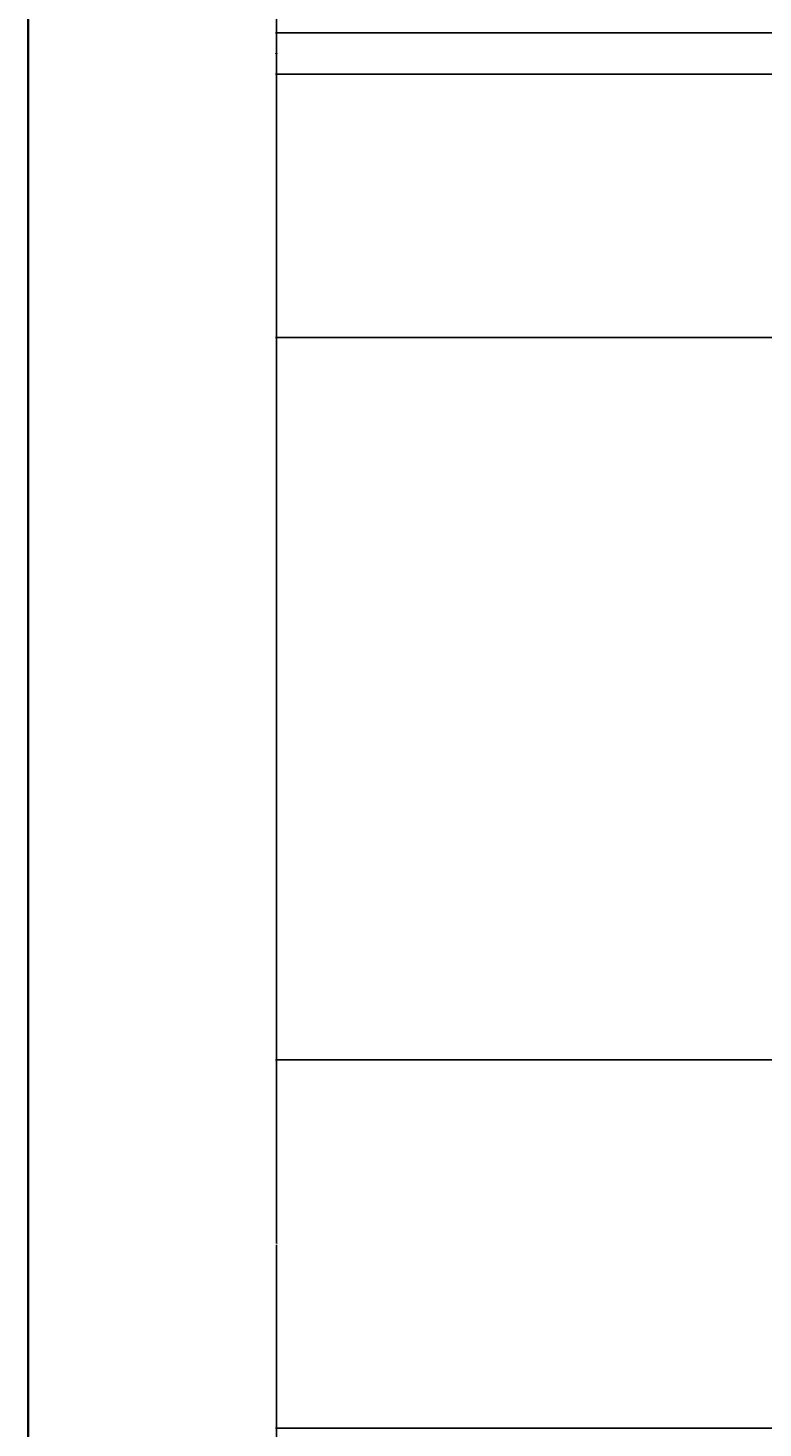
# Model space of a CAD drawing. Units: inches. Extents: x 1355 to 2746, y 1171 to 2751.
# Tile 5 of 24: x 1355 to 1511, y 1686 to 1983. Entities that reach past the tile are written whole.
import ezdxf

# ---------------------------------------------------------------- set-up
doc = ezdxf.new("R2010")
doc.units = ezdxf.units.IN
doc.layers.add('A-ANNO-DIMS', color=2, linetype='Continuous', lineweight=18)
doc.layers.add('A-ANNO-TTLB', color=7, linetype='Continuous', lineweight=35)
doc.styles.get("Standard").update_dxf_attribs({"font": 'arial.ttf'})
doc.dimstyles.get("Standard").update_dxf_attribs({"dimtxt": 0.18, "dimasz": 0.18, "dimexe": 0.18, "dimexo": 0.0625, "dimgap": 0.09, "dimtad": 0, "dimtih": 1, "dimtoh": 1, "dimdec": 4, "dimzin": 0, "dimdsep": 46, "dimtxsty": 'Standard', "dimcen": 0.09, "dimadec": 0, "dimazin": 0, "dimtfac": 1, "dimtdec": 4, "dimtofl": 0, "dimtmove": 0, "dimatfit": 3, "dimfxl": 1, "dimtolj": 1, "dimtzin": 0, "dimarcsym": 0})

# ---------------------------------------------------------------- blocks, each defined once
blk = doc.blocks.new('*D96')
at = {"layer": 'A-ANNO-DIMS', "color": 0, "lineweight": -2, "transparency": 16777216}
for p, q in [((1514.65, 2139.3), (1407.53, 2139.3)), ((1407.71, 2139.12), (1407.71, 1725.48)), ((1407.71, 1311.48), (1407.71, 1725.12)), ((1514.65, 1311.3), (1407.53, 1311.3))]:
    blk.add_line(p, q, dxfattribs=at)
at = {"layer": 'A-ANNO-DIMS', "color": 0, "transparency": 16777216}
for points in [[(1407.68, 2139.12), (1407.74, 2139.12), (1407.71, 2139.3)], [(1407.68, 1311.48), (1407.74, 1311.48), (1407.71, 1311.3)]]:
    blk.add_solid(points, dxfattribs=at)
at = {"layer": 'Defpoints', "color": 0, "transparency": 16777216}
for p in [(1407.71, 2139.3), (1514.71, 2139.3), (1514.71, 1311.3)]:
    blk.add_point(p, dxfattribs=at)
at = {"layer": 'A-ANNO-DIMS', "color": 0, "transparency": 16777216, "insert": (1407.71, 1725.3), "char_height": 0.18, "attachment_point": 5}
blk.add_mtext('\\A1;828', dxfattribs=at)
blk = doc.blocks.new('*D102')
at = {"layer": 'A-ANNO-DIMS', "color": 0, "lineweight": -2, "transparency": 16777216}
for p, q in [((2089.33, 1764.3), (1407.53, 1764.3)), ((1407.71, 1764.12), (1407.71, 1725.48)), ((1407.71, 1686.48), (1407.71, 1725.12)), ((2089.33, 1686.3), (1407.53, 1686.3))]:
    blk.add_line(p, q, dxfattribs=at)
at = {"layer": 'A-ANNO-DIMS', "color": 0, "transparency": 16777216}
for points in [[(1407.68, 1764.12), (1407.74, 1764.12), (1407.71, 1764.3)], [(1407.68, 1686.48), (1407.74, 1686.48), (1407.71, 1686.3)]]:
    blk.add_solid(points, dxfattribs=at)
at = {"layer": 'Defpoints', "color": 0, "transparency": 16777216}
for p in [(1407.71, 1764.3), (2089.39, 1764.3), (2089.39, 1686.3)]:
    blk.add_point(p, dxfattribs=at)
at = {"layer": 'A-ANNO-DIMS', "color": 0, "transparency": 16777216, "insert": (1407.71, 1725.3), "char_height": 0.18, "attachment_point": 5}
blk.add_mtext('\\A1;78', dxfattribs=at)
blk = doc.blocks.new('*D103')
at = {"layer": 'A-ANNO-DIMS', "color": 0, "lineweight": -2, "transparency": 16777216}
for p, q in [((2089.33, 1917.3), (1407.53, 1917.3)), ((1407.71, 1917.12), (1407.71, 1840.98)), ((1407.71, 1764.48), (1407.71, 1840.62)), ((2089.33, 1764.3), (1407.53, 1764.3))]:
    blk.add_line(p, q, dxfattribs=at)
at = {"layer": 'A-ANNO-DIMS', "color": 0, "transparency": 16777216}
for points in [[(1407.68, 1917.12), (1407.74, 1917.12), (1407.71, 1917.3)], [(1407.68, 1764.48), (1407.74, 1764.48), (1407.71, 1764.3)]]:
    blk.add_solid(points, dxfattribs=at)
at = {"layer": 'Defpoints', "color": 0, "transparency": 16777216}
for p in [(1407.71, 1917.3), (2089.39, 1917.3), (2089.39, 1764.3)]:
    blk.add_point(p, dxfattribs=at)
at = {"layer": 'A-ANNO-DIMS', "color": 0, "transparency": 16777216, "insert": (1407.71, 1840.8), "char_height": 0.18, "attachment_point": 5}
blk.add_mtext('\\A1;153', dxfattribs=at)
blk = doc.blocks.new('*D104')
at = {"layer": 'A-ANNO-DIMS', "color": 0, "lineweight": -2, "transparency": 16777216}
for p, q in [((2089.33, 1986.3), (1407.53, 1986.3)), ((1407.71, 1986.12), (1407.71, 1951.98)), ((1407.71, 1917.48), (1407.71, 1951.62)), ((2089.33, 1917.3), (1407.53, 1917.3))]:
    blk.add_line(p, q, dxfattribs=at)
at = {"layer": 'A-ANNO-DIMS', "color": 0, "transparency": 16777216}
for points in [[(1407.68, 1986.12), (1407.74, 1986.12), (1407.71, 1986.3)], [(1407.68, 1917.48), (1407.74, 1917.48), (1407.71, 1917.3)]]:
    blk.add_solid(points, dxfattribs=at)
at = {"layer": 'Defpoints', "color": 0, "transparency": 16777216}
for p in [(1407.71, 1986.3), (2089.39, 1986.3), (2089.39, 1917.3)]:
    blk.add_point(p, dxfattribs=at)
at = {"layer": 'A-ANNO-DIMS', "color": 0, "transparency": 16777216, "insert": (1407.71, 1951.8), "char_height": 0.18, "attachment_point": 5}
blk.add_mtext('\\A1;69', dxfattribs=at)
blk = doc.blocks.new('*D107')
at = {"layer": 'A-ANNO-DIMS', "color": 0, "lineweight": -2, "transparency": 16777216}
for p, q in [((2089.33, 1686.3), (1407.53, 1686.3)), ((1407.71, 1686.12), (1407.71, 1622.26)), ((1407.71, 1558.03), (1407.71, 1621.89)), ((2031.09, 1557.85), (1407.53, 1557.85))]:
    blk.add_line(p, q, dxfattribs=at)
at = {"layer": 'A-ANNO-DIMS', "color": 0, "transparency": 16777216}
for points in [[(1407.68, 1686.12), (1407.74, 1686.12), (1407.71, 1686.3)], [(1407.68, 1558.03), (1407.74, 1558.03), (1407.71, 1557.85)]]:
    blk.add_solid(points, dxfattribs=at)
at = {"layer": 'Defpoints', "color": 0, "transparency": 16777216}
for p in [(1407.71, 1686.3), (2089.39, 1686.3), (2031.15, 1557.85)]:
    blk.add_point(p, dxfattribs=at)
at = {"layer": 'A-ANNO-DIMS', "color": 0, "transparency": 16777216, "insert": (1407.71, 1622.07), "char_height": 0.18, "attachment_point": 5}
blk.add_mtext('\\A1;128.46', dxfattribs=at)
blk = doc.blocks.new('*D138')
at = {"layer": 'A-ANNO-DIMS', "color": 0, "lineweight": -2, "transparency": 16777216}
for p, q in [((1523.65, 1981.8), (1407.53, 1981.8)), ((1407.71, 1981.62), (1407.71, 1977.64)), ((1407.71, 1973.29), (1407.71, 1977.28)), ((1523.65, 1973.11), (1407.53, 1973.11))]:
    blk.add_line(p, q, dxfattribs=at)
at = {"layer": 'A-ANNO-DIMS', "color": 0, "transparency": 16777216}
for points in [[(1407.68, 1981.62), (1407.74, 1981.62), (1407.71, 1981.8)], [(1407.68, 1973.29), (1407.74, 1973.29), (1407.71, 1973.11)]]:
    blk.add_solid(points, dxfattribs=at)
at = {"layer": 'Defpoints', "color": 0, "transparency": 16777216}
for p in [(1407.71, 1981.8), (1523.71, 1981.8), (1523.71, 1973.11)]:
    blk.add_point(p, dxfattribs=at)
at = {"layer": 'A-ANNO-DIMS', "color": 0, "transparency": 16777216, "insert": (1407.71, 1977.46), "char_height": 0.18, "attachment_point": 5}
blk.add_mtext('\\A1;8.688', dxfattribs=at)

msp = doc.modelspace()

# ---------------------------------------------------------------- linework, layer by layer
at = {"layer": 'A-ANNO-TTLB'}
msp.add_lwpolyline([(1355.0901, 2751.4741), (2746.1804, 2751.4741), (2746.1804, 1182.883), (1355.0901, 1182.883)], close=True, dxfattribs=at)

# ---------------------------------------------------------------- dimensions: what is measured, and where the dimension line sits
at = {"layer": 'A-ANNO-DIMS'}
for base, p1, p2, override, picture, middle in [((1407.7083, 2139.3018), (1514.7083, 1311.3018), (1514.7083, 2139.3018), {"dimdec": 0, "dimlfac": 1, "dimrnd": 0, "dimzin": 0, "dimdsep": 46, "dimlunit": 2}, '*D96', (1407.7083, 1725.3018)), ((1407.7083, 1986.3018), (2089.3909, 1917.3018), (2089.3909, 1986.3018), {"dimdec": 0, "dimlfac": 1, "dimrnd": 0, "dimzin": 0, "dimdsep": 46, "dimlunit": 2}, '*D104', (1407.7083, 1951.8018)), ((1407.7083, 1981.8018), (1523.7077, 1973.1139), (1523.7083, 1981.8018), {"dimdec": 3, "dimlfac": 1, "dimrnd": 0, "dimzin": 0, "dimdsep": 46, "dimlunit": 2}, '*D138', (1407.7083, 1977.4578)), ((1407.7083, 1917.3018), (2089.3909, 1764.3018), (2089.3909, 1917.3018), {"dimdec": 0, "dimlfac": 1, "dimrnd": 0, "dimzin": 0, "dimdsep": 46, "dimlunit": 2}, '*D103', (1407.7083, 1840.8018)), ((1407.7083, 1764.3018), (2089.3909, 1686.3018), (2089.3909, 1764.3018), {"dimdec": 0, "dimlfac": 1, "dimrnd": 0, "dimzin": 0, "dimdsep": 46, "dimlunit": 2}, '*D102', (1407.7083, 1725.3018)), ((1407.7083, 1686.3018), (2031.1535, 1557.845), (2089.3909, 1686.3018), {"dimdec": 2, "dimlfac": 1, "dimrnd": 0, "dimzin": 0, "dimdsep": 46, "dimlunit": 2}, '*D107', (1407.7083, 1622.0734))]:
    dim = msp.add_linear_dim(base=base, p1=p1, p2=p2, angle=90, dimstyle='Standard', override=override, dxfattribs=at)
    dim.commit()
    dim.dimension.update_dxf_attribs({"geometry": picture, "text_midpoint": middle})

doc.saveas('drawing.dxf')
